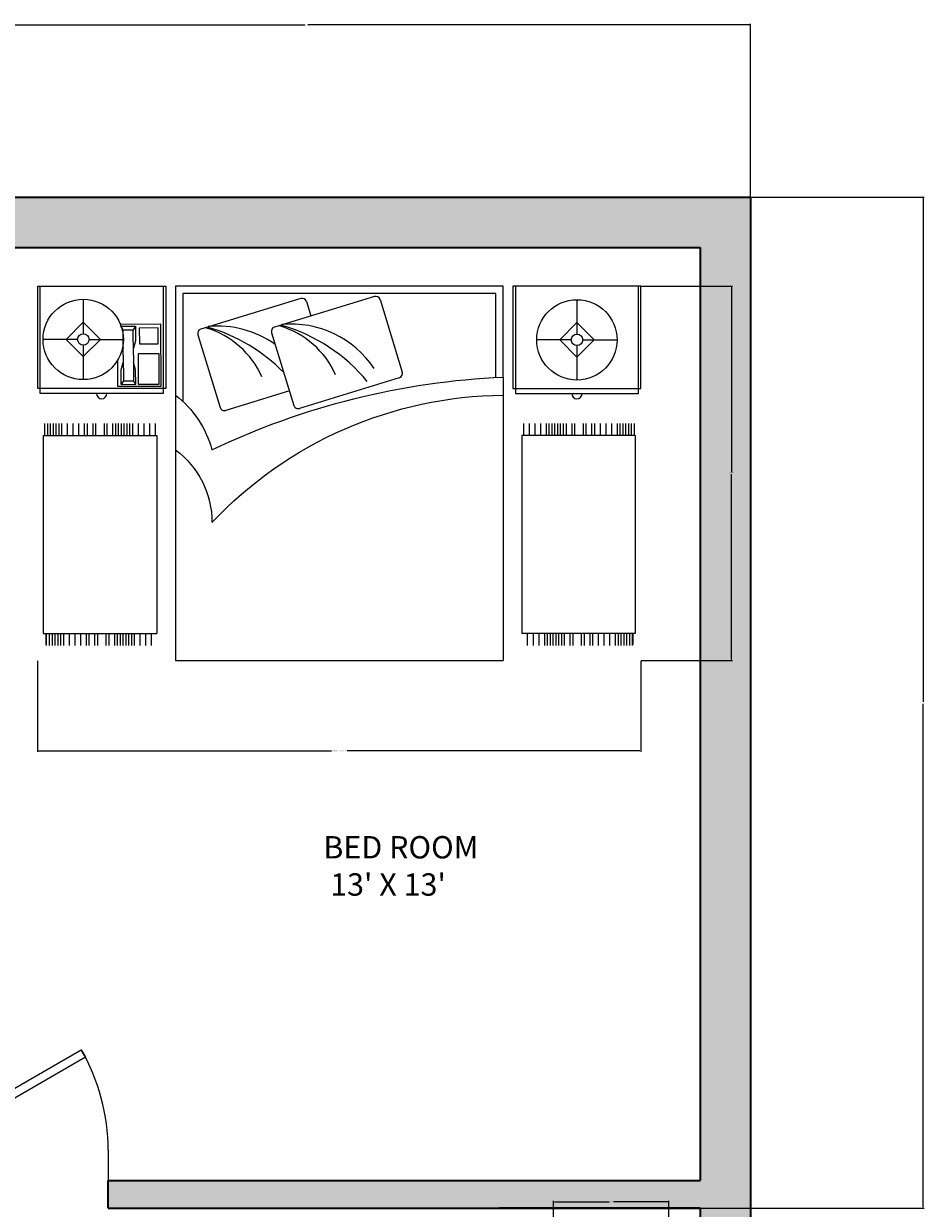
# Model space of a CAD drawing. Units: inches. Extents: x -30 to 437, y -29 to 647.
# Tile 15 of 15: x 276 to 437, y 435 to 647. Entities that reach past the tile are written whole.
import ezdxf

# ---------------------------------------------------------------- set-up
doc = ezdxf.new("R2010")
doc.units = ezdxf.units.IN
doc.header["$MEASUREMENT"] = 0
for name, color, linetype, lineweight in [('A-ANNO-DIMS', 2, 'Continuous', 18), ('A-AREA-IDEN', 7, 'Continuous', 18), ('A-WALL', 7, 'Continuous', 35), ('bedroom', 120, 'Continuous', 18), ('doors', 40, 'Continuous', 25)]:
    doc.layers.add(name, color=color, linetype=linetype, lineweight=lineweight)
doc.layers.add('A-WALL-PATT', color=251, linetype='Continuous', lineweight=13, true_color=0x636466)
doc.styles.get("Standard").update_dxf_attribs({"font": 'arial.ttf'})
doc.dimstyles.get("Standard").update_dxf_attribs({"dimtxt": 0.18, "dimasz": 0.18, "dimexe": 0.18, "dimexo": 0.0625, "dimgap": 0.09, "dimtad": 0, "dimtih": 1, "dimtoh": 1, "dimdec": 4, "dimzin": 0, "dimdsep": 46, "dimtxsty": 'Standard', "dimcen": 0.09, "dimadec": 0, "dimazin": 0, "dimtfac": 1, "dimtdec": 4, "dimtofl": 0, "dimtmove": 0, "dimatfit": 3, "dimfxl": 1, "dimtolj": 1, "dimtzin": 0, "dimarcsym": 0})

# ---------------------------------------------------------------- blocks, each defined once
blk = doc.blocks.new('3')
for p, q in [((185.8665, 224.6766), (185.8665, 225.2363)), ((185.8665, 225.2363), (186.566, 225.2363)), ((185.8805, 224.6487), (185.8805, 225.2363)), ((186.552, 225.2363), (186.552, 224.6487)), ((186.566, 225.2363), (186.566, 224.6766)), ((186.6199, 225.2363), (186.6199, 224.6399)), ((188.4089, 225.2363), (186.6199, 225.2363)), ((188.4089, 224.7393), (188.4089, 225.2363)), ((188.4627, 225.2363), (188.4627, 224.6766)), ((189.1623, 225.2363), (188.4627, 225.2363)), ((188.4767, 225.2363), (188.4767, 224.6486)), ((189.1483, 224.6486), (189.1483, 225.2363)), ((189.1623, 224.6766), (189.1623, 225.2363)), ((186.1157, 225.1643), (186.1157, 224.9763)), ((187.3034, 225.1683), (186.7581, 225.0015)), ((187.7059, 225.1793), (187.1607, 225.0124)), ((187.737, 225.1628), (187.8585, 224.7657)), ((188.8125, 225.1618), (188.8125, 224.9738)), ((187.3344, 225.1518), (187.3586, 225.073)), ((186.0216, 224.9449), (186.1157, 225.0389)), ((186.1157, 225.0389), (186.2097, 224.9449)), ((188.8125, 225.0365), (188.7185, 224.9424)), ((188.9065, 224.9424), (188.8125, 225.0365)), ((186.5397, 225.0274), (186.3193, 225.0266)), ((186.3215, 225.0167), (186.4008, 225.017)), ((186.3334, 224.9969), (186.3215, 225.0167)), ((186.3334, 224.9969), (186.389, 224.9971)), ((186.334, 224.858), (186.3334, 224.9969)), ((186.4008, 225.017), (186.389, 224.9971)), ((186.3895, 224.8582), (186.389, 224.9971)), ((186.4008, 225.017), (186.4011, 224.9376)), ((186.5409, 224.6901), (186.5397, 225.0274)), ((186.7416, 224.9704), (186.8631, 224.5734)), ((187.1442, 224.9814), (187.2657, 224.5843)), ((186.0843, 224.9449), (185.8963, 224.9449)), ((186.1157, 224.8509), (186.0216, 224.9449)), ((186.2097, 224.9449), (186.1157, 224.8509)), ((186.1157, 224.9136), (186.1157, 224.7256)), ((186.147, 224.9449), (186.335, 224.9449)), ((186.3314, 224.9055), (186.3338, 224.8977)), ((186.4011, 224.9376), (186.3894, 224.8979)), ((188.7812, 224.9424), (188.5931, 224.9424)), ((188.7185, 224.9424), (188.8125, 224.8484)), ((188.8125, 224.8484), (188.9065, 224.9424)), ((188.8125, 224.9111), (188.8125, 224.723)), ((188.8438, 224.9424), (189.0319, 224.9424)), ((186.334, 224.858), (186.3345, 224.7191)), ((186.3895, 224.8582), (186.39, 224.7193)), ((186.3023, 224.8297), (186.3029, 224.6892)), ((186.3224, 224.7786), (186.3341, 224.8183)), ((186.3227, 224.6992), (186.3224, 224.7786)), ((186.4017, 224.7789), (186.3897, 224.8185)), ((186.402, 224.6995), (186.4017, 224.7789)), ((186.3345, 224.7191), (186.3227, 224.6992)), ((186.3345, 224.7191), (186.39, 224.7193)), ((186.402, 224.6995), (186.39, 224.7193)), ((187.842, 224.7347), (187.2967, 224.5678)), ((188.4089, 224.7393), (188.4089, 223.1907)), ((186.566, 224.6766), (185.8665, 224.6766)), ((186.552, 224.6487), (185.8805, 224.6487)), ((186.3029, 224.6892), (186.5409, 224.6901)), ((186.3227, 224.6992), (186.402, 224.6995)), ((187.2416, 224.6632), (186.8942, 224.5569)), ((188.4627, 224.6766), (189.1623, 224.6766)), ((188.4767, 224.6486), (189.1483, 224.6486)), ((186.6199, 224.6399), (186.6199, 223.1907)), ((185.904, 224.4849, -0.9094), (185.904, 224.4204, -0.9094)), ((185.9195, 224.4849, -0.9094), (185.9195, 224.4204, -0.9094)), ((185.9195, 224.4849, -0.9094), (185.9195, 224.4204, -0.9094)), ((185.935, 224.4849, -0.9094), (185.935, 224.4204, -0.9094)), ((185.9505, 224.4849, -0.9094), (185.9505, 224.4204, -0.9094)), ((185.966, 224.4849, -0.9094), (185.966, 224.4204, -0.9094)), ((185.9815, 224.4849, -0.9094), (185.9815, 224.4204, -0.9094)), ((185.997, 224.4849, -0.9094), (185.997, 224.4204, -0.9094)), ((186.028, 224.4849, -0.9094), (186.028, 224.4204, -0.9094)), ((186.059, 224.4849, -0.9094), (186.059, 224.4204, -0.9094)), ((186.09, 224.4849, -0.9094), (186.09, 224.4204, -0.9094)), ((186.09, 224.4849, -0.9094), (186.09, 224.4204, -0.9094)), ((186.121, 224.4849, -0.9094), (186.121, 224.4204, -0.9094)), ((186.1365, 224.4849, -0.9094), (186.1365, 224.4204, -0.9094)), ((186.1675, 224.4849, -0.9094), (186.1675, 224.4204, -0.9094)), ((186.183, 224.4849, -0.9094), (186.183, 224.4204, -0.9094)), ((186.2295, 224.4849, -0.9094), (186.2295, 224.4204, -0.9094)), ((186.245, 224.4849, -0.9094), (186.245, 224.4204, -0.9094)), ((186.276, 224.4849, -0.9094), (186.276, 224.4204, -0.9094)), ((186.2915, 224.4849, -0.9094), (186.2915, 224.4204, -0.9094)), ((186.307, 224.4849, -0.9094), (186.307, 224.4204, -0.9094)), ((186.3225, 224.4849, -0.9094), (186.3225, 224.4204, -0.9094)), ((186.338, 224.4849, -0.9094), (186.338, 224.4204, -0.9094)), ((186.3535, 224.4849, -0.9094), (186.3535, 224.4204, -0.9094)), ((186.369, 224.4849, -0.9094), (186.369, 224.4204, -0.9094)), ((186.3845, 224.4849, -0.9094), (186.3845, 224.4204, -0.9094)), ((186.4155, 224.4849, -0.9094), (186.4155, 224.4204, -0.9094)), ((186.4465, 224.4849, -0.9094), (186.4465, 224.4204, -0.9094)), ((186.4775, 224.4849, -0.9094), (186.4775, 224.4204, -0.9094)), ((186.5085, 224.4849, -0.9094), (186.5085, 224.4204, -0.9094)), ((188.5202, 224.4849, -0.9094), (188.5202, 224.4204, -0.9094)), ((188.5512, 224.4849, -0.9094), (188.5512, 224.4204, -0.9094)), ((188.5822, 224.4849, -0.9094), (188.5822, 224.4204, -0.9094)), ((188.6132, 224.4849, -0.9094), (188.6132, 224.4204, -0.9094)), ((188.6442, 224.4849, -0.9094), (188.6442, 224.4204, -0.9094)), ((188.6597, 224.4849, -0.9094), (188.6597, 224.4204, -0.9094)), ((188.6752, 224.4849, -0.9094), (188.6752, 224.4204, -0.9094)), ((188.6907, 224.4849, -0.9094), (188.6907, 224.4204, -0.9094)), ((188.7062, 224.4849, -0.9094), (188.7062, 224.4204, -0.9094)), ((188.7217, 224.4849, -0.9094), (188.7217, 224.4204, -0.9094)), ((188.7372, 224.4849, -0.9094), (188.7372, 224.4204, -0.9094)), ((188.7527, 224.4849, -0.9094), (188.7527, 224.4204, -0.9094)), ((188.7837, 224.4849, -0.9094), (188.7837, 224.4204, -0.9094)), ((188.7992, 224.4849, -0.9094), (188.7992, 224.4204, -0.9094)), ((188.8457, 224.4849, -0.9094), (188.8457, 224.4204, -0.9094)), ((188.8612, 224.4849, -0.9094), (188.8612, 224.4204, -0.9094)), ((188.8922, 224.4849, -0.9094), (188.8922, 224.4204, -0.9094)), ((188.9077, 224.4849, -0.9094), (188.9077, 224.4204, -0.9094)), ((188.9387, 224.4849, -0.9094), (188.9387, 224.4204, -0.9094)), ((188.9387, 224.4849, -0.9094), (188.9387, 224.4204, -0.9094)), ((188.9697, 224.4849, -0.9094), (188.9697, 224.4204, -0.9094)), ((189.0007, 224.4849, -0.9094), (189.0007, 224.4204, -0.9094)), ((189.0317, 224.4849, -0.9094), (189.0317, 224.4204, -0.9094)), ((189.0472, 224.4849, -0.9094), (189.0472, 224.4204, -0.9094)), ((189.0627, 224.4849, -0.9094), (189.0627, 224.4204, -0.9094)), ((189.0782, 224.4849, -0.9094), (189.0782, 224.4204, -0.9094)), ((189.0937, 224.4849, -0.9094), (189.0937, 224.4204, -0.9094)), ((189.1092, 224.4849, -0.9094), (189.1092, 224.4204, -0.9094)), ((189.1092, 224.4849, -0.9094), (189.1092, 224.4204, -0.9094)), ((189.1247, 224.4849, -0.9094), (189.1247, 224.4204, -0.9094)), ((185.8974, 224.4204, -0.9094), (185.8974, 223.3378, -0.9094)), ((185.8974, 224.4204, -0.9094), (186.5174, 224.4204, -0.9094)), ((186.5174, 224.4204, -0.9094), (186.5174, 223.3378, -0.9094)), ((189.1313, 224.4204, -0.9094), (188.5113, 224.4204, -0.9094)), ((188.5113, 224.4204, -0.9094), (188.5113, 223.3378, -0.9094)), ((189.1313, 224.4204, -0.9094), (189.1313, 223.3378, -0.9094)), ((185.8974, 223.3378, -0.9094), (186.5174, 223.3378, -0.9094)), ((185.9114, 223.3378, -0.9094), (185.9114, 223.2789, -0.9094)), ((185.9114, 223.3378, -0.9094), (185.9114, 223.2789, -0.9094)), ((185.9114, 223.3378, -0.9094), (185.9114, 223.2789, -0.9094)), ((185.9138, 223.3378, -0.9094), (185.9138, 223.2732, -0.9094)), ((185.9293, 223.3378, -0.9094), (185.9293, 223.2732, -0.9094)), ((185.9293, 223.3378, -0.9094), (185.9293, 223.2732, -0.9094)), ((185.9448, 223.3378, -0.9094), (185.9448, 223.2732, -0.9094)), ((185.9603, 223.3378, -0.9094), (185.9603, 223.2732, -0.9094)), ((185.9758, 223.3378, -0.9094), (185.9758, 223.2732, -0.9094)), ((185.9913, 223.3378, -0.9094), (185.9913, 223.2732, -0.9094)), ((186.0068, 223.3378, -0.9094), (186.0068, 223.2732, -0.9094)), ((186.0378, 223.3378, -0.9094), (186.0378, 223.2732, -0.9094)), ((186.0688, 223.3378, -0.9094), (186.0688, 223.2732, -0.9094)), ((186.0998, 223.3378, -0.9094), (186.0998, 223.2732, -0.9094)), ((186.0998, 223.3378, -0.9094), (186.0998, 223.2732, -0.9094)), ((186.1308, 223.3378, -0.9094), (186.1308, 223.2732, -0.9094)), ((186.1463, 223.3378, -0.9094), (186.1463, 223.2732, -0.9094)), ((186.1773, 223.3378, -0.9094), (186.1773, 223.2732, -0.9094)), ((186.1928, 223.3378, -0.9094), (186.1928, 223.2732, -0.9094)), ((186.2393, 223.3378, -0.9094), (186.2393, 223.2732, -0.9094)), ((186.2548, 223.3378, -0.9094), (186.2548, 223.2732, -0.9094)), ((186.2858, 223.3378, -0.9094), (186.2858, 223.2732, -0.9094)), ((186.3013, 223.3378, -0.9094), (186.3013, 223.2732, -0.9094)), ((186.3168, 223.3378, -0.9094), (186.3168, 223.2732, -0.9094)), ((186.3323, 223.3378, -0.9094), (186.3323, 223.2732, -0.9094)), ((186.3478, 223.3378, -0.9094), (186.3478, 223.2732, -0.9094)), ((186.3633, 223.3378, -0.9094), (186.3633, 223.2732, -0.9094)), ((186.3788, 223.3378, -0.9094), (186.3788, 223.2732, -0.9094)), ((186.3943, 223.3378, -0.9094), (186.3943, 223.2732, -0.9094)), ((186.4253, 223.3378, -0.9094), (186.4253, 223.2732, -0.9094)), ((186.4563, 223.3378, -0.9094), (186.4563, 223.2732, -0.9094)), ((186.4873, 223.3378, -0.9094), (186.4873, 223.2732, -0.9094)), ((189.1313, 223.3378, -0.9094), (188.5113, 223.3378, -0.9094)), ((188.5414, 223.3378, -0.9094), (188.5414, 223.2732, -0.9094)), ((188.5724, 223.3378, -0.9094), (188.5724, 223.2732, -0.9094)), ((188.6034, 223.3378, -0.9094), (188.6034, 223.2732, -0.9094)), ((188.6344, 223.3378, -0.9094), (188.6344, 223.2732, -0.9094)), ((188.6499, 223.3378, -0.9094), (188.6499, 223.2732, -0.9094)), ((188.6654, 223.3378, -0.9094), (188.6654, 223.2732, -0.9094)), ((188.6809, 223.3378, -0.9094), (188.6809, 223.2732, -0.9094)), ((188.6964, 223.3378, -0.9094), (188.6964, 223.2732, -0.9094)), ((188.7119, 223.3378, -0.9094), (188.7119, 223.2732, -0.9094)), ((188.7274, 223.3378, -0.9094), (188.7274, 223.2732, -0.9094)), ((188.7429, 223.3378, -0.9094), (188.7429, 223.2732, -0.9094)), ((188.7739, 223.3378, -0.9094), (188.7739, 223.2732, -0.9094)), ((188.7894, 223.3378, -0.9094), (188.7894, 223.2732, -0.9094)), ((188.8359, 223.3378, -0.9094), (188.8359, 223.2732, -0.9094)), ((188.8514, 223.3378, -0.9094), (188.8514, 223.2732, -0.9094)), ((188.8824, 223.3378, -0.9094), (188.8824, 223.2732, -0.9094)), ((188.8979, 223.3378, -0.9094), (188.8979, 223.2732, -0.9094)), ((188.9289, 223.3378, -0.9094), (188.9289, 223.2732, -0.9094)), ((188.9289, 223.3378, -0.9094), (188.9289, 223.2732, -0.9094)), ((188.9599, 223.3378, -0.9094), (188.9599, 223.2732, -0.9094)), ((188.9909, 223.3378, -0.9094), (188.9909, 223.2732, -0.9094)), ((189.022, 223.3378, -0.9094), (189.022, 223.2732, -0.9094)), ((189.0375, 223.3378, -0.9094), (189.0375, 223.2732, -0.9094)), ((189.053, 223.3378, -0.9094), (189.053, 223.2732, -0.9094)), ((189.0685, 223.3378, -0.9094), (189.0685, 223.2732, -0.9094)), ((189.084, 223.3378, -0.9094), (189.084, 223.2732, -0.9094)), ((189.0995, 223.3378, -0.9094), (189.0995, 223.2732, -0.9094)), ((189.0995, 223.3378, -0.9094), (189.0995, 223.2732, -0.9094)), ((189.115, 223.3378, -0.9094), (189.115, 223.2732, -0.9094)), ((189.1173, 223.3378, -0.9094), (189.1173, 223.2789, -0.9094)), ((189.1173, 223.3378, -0.9094), (189.1173, 223.2789, -0.9094)), ((189.1173, 223.3378, -0.9094), (189.1173, 223.2789, -0.9094)), ((186.6199, 223.1907), (188.4089, 223.1907))]:
    blk.add_line(p, q)
blk.add_lwpolyline([(188.3691, 224.7374), (188.3691, 225.1965), (186.6596, 225.1965), (186.6596, 224.606)])
for points in [[(186.4217, 225.0072), (186.422, 224.9199), (186.5252, 224.9202), (186.5249, 225.0075)], [(186.4153, 224.8663), (186.4159, 224.6996), (186.531, 224.7), (186.5304, 224.8667)]]:
    blk.add_lwpolyline(points, close=True)
for points in [[(186.6199, 224.6399, -0.162278), (186.8186, 224.3418, -0.100664), (188.4089, 224.7393, -0.100664)], [(186.6199, 224.3418, -0.236068), (186.8186, 223.9442, -0.205258), (188.4089, 224.6399, -0.205258)]]:
    blk.add_lwpolyline(points, format="xyb")
for centre, radius in [((186.1157, 224.9449), 0.2194), ((188.8125, 224.9424), 0.2194), ((186.1157, 224.9449), 0.0313), ((188.8125, 224.9424), 0.0313)]:
    blk.add_circle(centre, radius)
for centre, radius, start, end in [((187.3107, 225.1446), 0.0248, 17.0142, 107.0142), ((187.7132, 225.1555), 0.0248, 17.0142, 107.0142), ((186.7654, 224.9777), 0.0248, 107.0142, 197.0142), ((186.6474, 224.5408), 0.4873, 24.22087, 73.06906), ((186.8477, 224.4712), 0.5468, 54.68511, 95.16051), ((186.5359, 224.1054), 0.9426, 44.27274, 73.71889), ((187.1679, 224.9887), 0.0248, 107.0142, 197.0142), ((187.0499, 224.5517), 0.4873, 24.22087, 73.06906), ((187.2502, 224.4821), 0.5468, 33.78007, 95.16051), ((186.9385, 224.1164), 0.9426, 39.40233, 73.71889), ((187.8347, 224.7585), 0.0248, 287.0142, 17.0142), ((186.2163, 224.6487), 0.028, 180, 0), ((188.8125, 224.6486), 0.028, 180, 0), ((187.2894, 224.5916), 0.0248, 197.0142, 287.0142), ((186.8869, 224.5806), 0.0248, 197.0142, 287.0142)]:
    blk.add_arc(centre, radius, start, end)
blk = doc.blocks.new('*U6')
for p, q in [((0, 0), (0, -6)), ((40, 0), (40, -6))]:
    blk.add_line(p, q)
blk.add_lwpolyline([(0, 0), (34.64, 20), (35.52, 18.48), (0.87, -1.52)], close=True)
blk.add_arc((0, 0), 40, 0, 30)
blk = doc.blocks.new('*D11')
at = {"layer": 'A-ANNO-DIMS', "color": 0, "lineweight": -2, "transparency": 16777216}
for p, q in [((278.06, 532.56), (278.06, 516.24)), ((386.06, 532.56), (386.06, 516.24)), ((278.24, 516.42), (330.68, 516.42)), ((385.88, 516.42), (333.45, 516.42))]:
    blk.add_line(p, q, dxfattribs=at)
at = {"layer": 'A-ANNO-DIMS', "color": 0, "transparency": 16777216}
for points in [[(278.24, 516.45), (278.24, 516.39), (278.06, 516.42)], [(385.88, 516.45), (385.88, 516.39), (386.06, 516.42)]]:
    blk.add_solid(points, dxfattribs=at)
at = {"layer": 'Defpoints', "color": 0, "transparency": 16777216}
for p in [(278.06, 532.62), (386.06, 532.62), (386.06, 516.42)]:
    blk.add_point(p, dxfattribs=at)
at = {"layer": 'A-ANNO-DIMS', "color": 0, "transparency": 16777216, "insert": (332.06, 516.42), "char_height": 0.18, "attachment_point": 5}
blk.add_mtext('\\A1;BED GROUP 108 TYP.', dxfattribs=at)
blk = doc.blocks.new('*D12')
at = {"layer": 'A-ANNO-DIMS', "color": 0, "lineweight": -2, "transparency": 16777216}
for p, q in [((386.12, 599.65), (402.44, 599.65)), ((402.26, 599.47), (402.26, 566.32)), ((402.26, 532.8), (402.26, 565.95)), ((386.12, 532.62), (402.44, 532.62))]:
    blk.add_line(p, q, dxfattribs=at)
at = {"layer": 'A-ANNO-DIMS', "color": 0, "transparency": 16777216}
for points in [[(402.23, 599.47), (402.29, 599.47), (402.26, 599.65)], [(402.23, 532.8), (402.29, 532.8), (402.26, 532.62)]]:
    blk.add_solid(points, dxfattribs=at)
at = {"layer": 'Defpoints', "color": 0, "transparency": 16777216}
for p in [(386.06, 599.65), (402.26, 599.65), (386.06, 532.62)]:
    blk.add_point(p, dxfattribs=at)
at = {"layer": 'A-ANNO-DIMS', "color": 0, "transparency": 16777216, "insert": (402.26, 566.14), "char_height": 0.18, "attachment_point": 5}
blk.add_mtext('\\A1;67 TYP.', dxfattribs=at)
blk = doc.blocks.new('*D29')
at = {"layer": 'A-ANNO-DIMS', "color": 0, "lineweight": -2, "transparency": 16777216}
for p, q in [((246.67, 606.61), (246.67, 646.63)), ((246.85, 646.45), (325.89, 646.45)), ((405.49, 646.45), (326.45, 646.45)), ((405.67, 615.61), (405.67, 646.63))]:
    blk.add_line(p, q, dxfattribs=at)
at = {"layer": 'A-ANNO-DIMS', "color": 0, "transparency": 16777216}
for points in [[(246.85, 646.48), (246.85, 646.42), (246.67, 646.45)], [(405.49, 646.48), (405.49, 646.42), (405.67, 646.45)]]:
    blk.add_solid(points, dxfattribs=at)
at = {"layer": 'Defpoints', "color": 0, "transparency": 16777216}
for p in [(405.67, 646.45), (405.67, 615.55), (246.67, 606.55)]:
    blk.add_point(p, dxfattribs=at)
at = {"layer": 'A-ANNO-DIMS', "color": 0, "transparency": 16777216, "insert": (326.17, 646.45), "char_height": 0.18, "attachment_point": 5}
blk.add_mtext('\\A1;159', dxfattribs=at)
blk = doc.blocks.new('*D40')
at = {"layer": 'A-ANNO-DIMS', "color": 0, "lineweight": -2, "transparency": 16777216}
for p, q in [((405.74, 615.55), (436.75, 615.55)), ((436.57, 615.37), (436.57, 525.23)), ((436.57, 434.73), (436.57, 524.87)), ((396.74, 434.55), (436.75, 434.55))]:
    blk.add_line(p, q, dxfattribs=at)
at = {"layer": 'A-ANNO-DIMS', "color": 0, "transparency": 16777216}
for points in [[(436.54, 615.37), (436.6, 615.37), (436.57, 615.55)], [(436.54, 434.73), (436.6, 434.73), (436.57, 434.55)]]:
    blk.add_solid(points, dxfattribs=at)
at = {"layer": 'Defpoints', "color": 0, "transparency": 16777216}
for p in [(405.67, 615.55), (436.57, 615.55), (396.67, 434.55)]:
    blk.add_point(p, dxfattribs=at)
at = {"layer": 'A-ANNO-DIMS', "color": 0, "transparency": 16777216, "insert": (436.57, 525.05), "char_height": 0.18, "attachment_point": 5}
blk.add_mtext('\\A1;181', dxfattribs=at)
blk = doc.blocks.new('*D47')
at = {"layer": 'A-ANNO-DIMS', "color": 0, "lineweight": -2, "transparency": 16777216}
for p, q in [((370.39, 404.84), (370.39, 435.86)), ((370.57, 435.68), (380.34, 435.68)), ((390.89, 435.68), (381.13, 435.68)), ((391.07, 404.84), (391.07, 435.86))]:
    blk.add_line(p, q, dxfattribs=at)
at = {"layer": 'A-ANNO-DIMS', "color": 0, "transparency": 16777216}
for points in [[(370.57, 435.71), (370.57, 435.65), (370.39, 435.68)], [(390.89, 435.71), (390.89, 435.65), (391.07, 435.68)]]:
    blk.add_solid(points, dxfattribs=at)
at = {"layer": 'Defpoints', "color": 0, "transparency": 16777216}
for p in [(391.07, 435.68), (370.39, 404.78), (391.07, 404.78)]:
    blk.add_point(p, dxfattribs=at)
at = {"layer": 'A-ANNO-DIMS', "color": 0, "transparency": 16777216, "insert": (380.73, 435.68), "char_height": 0.18, "attachment_point": 5}
blk.add_mtext('\\A1;20.68', dxfattribs=at)

msp = doc.modelspace()

# ---------------------------------------------------------------- hatches: boundary and pattern name
at = {"layer": 'A-WALL-PATT'}
h = msp.add_hatch(color=256, dxfattribs=at)
h.dxf.hatch_style = 1
h.paths.add_polyline_path([(393.6054, 183.2352), (369.6054, 183.2352), (369.6054, 213.2352), (393.6054, 213.2352), (393.6054, 207.2352), (394.6054, 207.2352), (394.6054, 211.2352), (395.6054, 211.2352), (395.6054, 185.2352), (394.6054, 185.2352), (394.6054, 189.2352), (393.6054, 189.2352)], flags=0)
h.paths.add_polyline_path([(384.6054, 189.2352, -1), (390.6054, 189.2352, -1)], flags=0)
h.paths.add_polyline_path([(385.6054, 189.2352, -1), (389.6054, 189.2352, -1)], flags=0)
h.paths.add_polyline_path([(374.6054, 189.2352, -1), (382.6054, 189.2352, -1)], flags=0)
h.paths.add_polyline_path([(386.6054, 189.2352, -1), (388.6054, 189.2352, -1)], flags=0)
h.paths.add_polyline_path([(375.6054, 189.2352, -1), (381.6054, 189.2352, -1)], flags=0)
h.paths.add_polyline_path([(376.6054, 189.2352, -1), (380.6054, 189.2352, -1)], flags=0)
h.paths.add_polyline_path([(377.6054, 189.2352, -1), (379.6054, 189.2352, -1)], flags=0)
h.paths.add_polyline_path([(390.6054, 195.2352), (374.6054, 195.2352), (374.6054, 201.2352), (390.6054, 201.2352)], flags=0)
h.paths.add_polyline_path([(389.6054, 196.2352), (375.6054, 196.2352), (375.6054, 200.2352), (389.6054, 200.2352)], flags=0)
h.paths.add_polyline_path([(383.6054, 207.2352, -1), (391.6054, 207.2352, -1)], flags=0)
h.paths.add_polyline_path([(384.6054, 207.2352, -1), (390.6054, 207.2352, -1)], flags=0)
h.paths.add_polyline_path([(385.6054, 207.2352, -1), (389.6054, 207.2352, -1)], flags=0)
h.paths.add_polyline_path([(386.6054, 207.2352, -1), (388.6054, 207.2352, -1)], flags=0)
h.paths.add_polyline_path([(375.6054, 207.2352, -1), (381.6054, 207.2352, -1)], flags=0)
h.paths.add_polyline_path([(376.6054, 207.2352, -1), (380.6054, 207.2352, -1)], flags=0)
h.paths.add_polyline_path([(377.6054, 207.2352, -1), (379.6054, 207.2352, -1)], flags=0)
h.paths.add_polyline_path([(305.5437, 160.3663, -0.41421356), (304.0437, 158.8663), (271.0437, 158.8663, -0.41421356), (269.5437, 160.3663), (269.5437, 178.3663, -0.41421356), (271.0437, 179.8663), (304.0437, 179.8663, -0.41421356), (305.5437, 178.3663)], flags=0)
h.paths.add_polyline_path([(304.0437, 165.3663, -0.41421356), (303.0437, 164.3663), (289.2937, 164.3663, -0.41421356), (288.2937, 165.3663), (288.2937, 177.3663, -0.41421356), (289.2937, 178.3663), (303.0437, 178.3663, -0.41421356), (304.0437, 177.3663)], flags=0)
h.paths.add_polyline_path([(296.5437, 171.3663, -1), (295.5437, 171.3663, -1)], flags=0)
h.paths.add_polyline_path([(286.7937, 165.3663, -0.41421356), (285.7937, 164.3663), (272.0437, 164.3663, -0.41421356), (271.0437, 165.3663), (271.0437, 177.3663, -0.41421356), (272.0437, 178.3663), (285.7937, 178.3663, -0.41421356), (286.7937, 177.3663)], flags=0)
h.paths.add_polyline_path([(279.5437, 171.3663, -1), (278.5437, 171.3663, -1)], flags=0)
h.paths.add_polyline_path([(360.6737, 290.5474), (360.6737, 300.5474), (396.6737, 300.5474), (396.6737, 290.5474)], flags=0)
h.paths.add_polyline_path([(259.6737, 124.5474), (259.6737, 114.5474), (171.6737, 114.5474), (171.6737, 124.5474)], flags=0)
h.paths.add_polyline_path([(288.0737, 215.3705), (286.7097, 214.583), (268.7097, 245.7599), (270.0737, 246.5474)], flags=0)
h.paths.add_polyline_path([(259.6737, 168.5474), (256.6737, 168.5474), (256.6737, 173.5474), (256.6737, 179.0224), (255.8753, 177.6395), (224.2956, 195.872, 0.12053744), (220.1737, 179.0224, 0.12053744), (216.0518, 195.872), (184.4721, 177.6395), (183.6737, 179.0224), (215.2836, 197.2724), (216.0821, 195.8895), (216.0518, 195.872, -0.12053744), (220.1737, 179.0224, -0.12053744), (224.2956, 195.872), (224.2653, 195.8895), (225.0638, 197.2724), (256.6737, 179.0224), (256.6737, 173.5474), (259.6737, 173.5474)], flags=0)
h.paths.add_polyline_path([(386.7943, 325.4601), (372.6871, 325.4601), (372.6871, 339.5673), (386.7943, 339.5673)], flags=0)
h.paths.add_polyline_path([(359.5875, 343.7429), (357.7905, 343.7429), (357.7905, 327.9179), (359.3933, 327.9179, 0.41420885), (361.5302, 330.0549), (361.5302, 341.8434, 0.41436161)], flags=0)
h.paths.add_polyline_path([(341.7887, 323.1235, -0.11921667), (340.7839, 323.1235)], flags=0)
h.paths.add_polyline_path([(379.6332, 328.8632), (379.6332, 332.2699), (376.0992, 332.2699, 0.39427733)], flags=0)
h.paths.add_polyline_path([(375.5299, 332.459, -1), (383.8511, 332.459, -1)], flags=0)
h.paths.add_polyline_path([(388.9363, 344.7425), (372.5309, 344.7425, -0.41421356), (370.394, 346.8794), (370.394, 347.5594, -0.39085173), (372.3472, 349.7005, -0.43951011), (370.394, 351.4933), (370.394, 365.1894, -0.40305452), (372.2191, 367.1298, -0.41839453), (370.394, 368.9291), (370.394, 382.6251, -0.40885826), (372.2519, 384.5722, -0.42377324), (370.394, 386.3707), (370.394, 400.0667, -0.38660687), (372.1327, 402.0094), (372.531, 402.0094, -0.41421834), (370.394, 404.1464), (370.394, 404.7778, -0.41420891), (372.5309, 406.9147), (388.9363, 406.9147, -0.41421821), (391.0733, 404.7778), (391.0733, 346.8794, -0.41421356)], flags=0)
edge = h.paths.add_edge_path(flags=0)
edge.add_spline(control_points=[(349.3585, 363.204), (349.0859, 363.204), (348.8133, 363.2227), (348.2712, 363.2973), (348.0016, 363.3531), (347.3533, 363.5328), (346.9776, 363.6755), (346.2445, 364.0308), (345.887, 364.2432), (345.1953, 364.7329), (344.8611, 365.0101), (344.2197, 365.6237), (343.9125, 365.9603), (343.211, 366.8336), (342.8313, 367.3965), (342.1401, 368.6117), (341.8286, 369.2641), (341.2807, 370.64), (341.0443, 371.3636), (340.6522, 372.8619), (340.4964, 373.6367), (340.2695, 375.2158), (340.1983, 376.0203), (340.142, 377.6365), (340.157, 378.4483), (340.2729, 380.0567), (340.3738, 380.8533), (340.6589, 382.4093), (340.8432, 383.1686), (341.2906, 384.629), (341.5538, 385.3301), (342.1531, 386.6544), (342.4891, 387.2776), (343.2266, 388.4288), (343.6281, 388.9567), (344.4879, 389.9012), (344.9463, 390.3178), (345.7981, 390.9428), (346.182, 391.1771), (346.9712, 391.5648), (347.3766, 391.7182), (348.2004, 391.9387), (348.6189, 392.0058), (349.4588, 392.0508), (349.8801, 392.0288), (350.7146, 391.8966), (351.1278, 391.7865), (351.9366, 391.4822), (352.3323, 391.2882), (353.0989, 390.8223), (353.4699, 390.5504), (354.1819, 389.9355), (354.5229, 389.5924), (355.1706, 388.8418), (355.4772, 388.4343), (356.1315, 387.4422), (356.4671, 386.8397), (357.0692, 385.5581), (357.3356, 384.879), (357.7933, 383.4624), (357.9846, 382.725), (358.2875, 381.2112), (358.3992, 380.4349), (358.5404, 378.8643), (358.5699, 378.0699), (358.546, 376.4841), (358.4926, 375.6928), (358.3042, 374.1343), (358.1692, 373.3672), (357.8207, 371.8774), (357.6072, 371.1549), (357.1067, 369.7735), (356.8196, 369.1148), (356.1782, 367.8787), (355.8238, 367.3013), (355.0551, 366.244), (354.6408, 365.7641), (353.7607, 364.9161), (353.2948, 364.5481), (352.445, 364.0149), (352.0701, 363.822), (351.3034, 363.5117), (350.9116, 363.3943), (350.1325, 363.2418), (349.7455, 363.204), (349.3585, 363.204)], knot_values=[3.14159265, 3.14159265, 3.14159265, 3.14159265, 3.22691715, 3.22691715, 3.31224165, 3.31224165, 3.43426671, 3.43426671, 3.55629177, 3.55629177, 3.67831683, 3.67831683, 3.8003419, 3.8003419, 3.97157384, 3.97157384, 4.14280577, 4.14280577, 4.31403771, 4.31403771, 4.48526965, 4.48526965, 4.65650159, 4.65650159, 4.82773353, 4.82773353, 4.99896547, 4.99896547, 5.1701974, 5.1701974, 5.34142934, 5.34142934, 5.51266128, 5.51266128, 5.68389322, 5.68389322, 5.85512516, 5.85512516, 5.98669107, 5.98669107, 6.11825699, 6.11825699, 6.24982291, 6.24982291, 6.38138882, 6.38138882, 6.51295474, 6.51295474, 6.64452065, 6.64452065, 6.77608657, 6.77608657, 6.90765249, 6.90765249, 7.0392184, 7.0392184, 7.20701563, 7.20701563, 7.37481286, 7.37481286, 7.54261009, 7.54261009, 7.71040732, 7.71040732, 7.87820455, 7.87820455, 8.04600178, 8.04600178, 8.21379901, 8.21379901, 8.38159624, 8.38159624, 8.54939347, 8.54939347, 8.7171907, 8.7171907, 8.88498794, 8.88498794, 9.05278517, 9.05278517, 9.17820699, 9.17820699, 9.30362881, 9.30362881, 9.42477796, 9.42477796, 9.42477796, 9.42477796], degree=3, periodic=0)
edge.add_line((341.1696, 384.3006), (341.2012, 384.2808))
edge = h.paths.add_edge_path(flags=0)
edge.add_line((344.3353, 388.7801), (344.317, 388.7915))
edge.add_ellipse((349.3585, 377.6204), major_axis=(0, -13.7895), ratio=0.62186025, start_angle=-244.867444, end_angle=-124.769923)
h.paths.add_polyline_path([(163.6737, 163.1474), (132.4968, 145.1474), (131.7093, 146.5114), (162.8862, 164.5114)], flags=0)
h.paths.add_polyline_path([(366.4355, 409.0896, -0.41423669), (364.2985, 406.9525, -0.4913499), (361.5302, 408.8973), (361.5302, 420.6405, 0.41421356), (359.3932, 422.7775), (357.7905, 422.7775), (357.7905, 406.9525), (359.6317, 406.9525, 0.42741026), (361.5332, 408.9757, 0.39869469), (363.6672, 406.9525, 0.51958103), (366.4355, 409.0895)], flags=0)
h.paths.add_polyline_path([(386.7943, 410.9671), (372.6871, 410.9671), (372.6871, 425.0742), (386.7943, 425.0742)], flags=0)
h.paths.add_polyline_path([(379.6332, 414.3701), (379.6332, 417.7768), (376.0992, 417.7768, 0.39427733)], flags=0)
h.paths.add_polyline_path([(375.5299, 417.966, -1), (383.8511, 417.966, -1)], flags=0)
h.paths.add_polyline_path([(150.0377, 351.583), (148.6737, 352.3705), (166.6737, 383.5474), (168.0377, 382.7599)], flags=0)
h.paths.add_polyline_path([(91.6737, 234.1974), (66.559, 219.6974), (65.9246, 220.7962), (91.0393, 235.2962)], flags=0)
h.paths.add_polyline_path([(255.4612, 443.5834), (254.6737, 444.9474), (285.8506, 462.9474), (286.6381, 461.5834)], flags=0)
h.paths.add_polyline_path([(176.2737, 394.5474), (158.2737, 425.7243), (159.6377, 426.5118), (177.6377, 395.3349)], flags=0)
h.paths.add_polyline_path([(243.6737, 439.5474), (243.0393, 438.4486), (217.9246, 452.9486), (218.559, 454.0474)], flags=0)
h.paths.add_polyline_path([(38.1264, 269.8429), (40.2408, 269.8429), (40.2408, 270.3508), (38.1264, 270.3508)], flags=0)
h.paths.add_polyline_path([(75.7157, 289.9439), (40.2408, 289.9439), (38.1264, 289.6524), (40.2408, 289.6524)], flags=0)
h.paths.add_polyline_path([(75.7157, 270.0846), (77.6447, 270.0846), (77.6697, 270.1626), (75.7175, 270.1626)], flags=0)
h.paths.add_polyline_path([(80.5373, 293.3002), (33.0467, 293.3002), (13.5054, 293.3002), (13.5054, 351.9244), (29.7898, 351.9244), (80.5373, 351.9244)], flags=0)
h.paths.add_polyline_path([(46.0261, 212.466, -0.50131678), (27.1651, 207.5106), (21.165, 209.5107), (21.165, 206.5107), (22.665, 206.5107), (22.665, 203.5107), (21.165, 203.5107), (21.165, 203.0107), (13.165, 203.0107), (13.165, 224.0107), (21.165, 224.0107), (21.165, 217.5107), (27.1649, 219.5106, -0.50132349), (46.0261, 214.5554, -0.13289091)], flags=0)
h.paths.add_polyline_path([(44.688, 211.8666, -0.48007965), (27.165, 209.5107), (27.165, 217.5107, -0.4800795), (44.688, 215.1547, -0.21500378)], flags=0)
h.paths.add_polyline_path([(19.415, 204.0107), (15.165, 204.0107, -0.41421356), (14.165, 204.7607), (14.165, 222.0107, -0.41421356), (14.915, 223.0107), (19.165, 223.0107, -0.41421356), (20.165, 222.2607), (20.165, 205.0107, -0.41421356)], flags=0)
h.paths.add_polyline_path([(32.7608, 269.0719), (31.8439, 269.0719), (31.8439, 268.6134), (13.5054, 268.6134), (13.5054, 291.5366), (31.8439, 291.5366), (32.7608, 291.0781), (32.7608, 280.9919, -1), (32.7608, 279.1581)], flags=0)
h.paths.add_polyline_path([(40.2408, 360.1436), (38.1264, 360.1436), (38.1264, 359.6357), (40.2408, 359.6357)], flags=0)
h.paths.add_polyline_path([(75.7157, 355.2807), (40.2408, 355.2807), (38.1264, 355.5722), (40.2408, 355.5722), (40.2408, 355.2807), (75.7157, 355.2807), (75.7157, 375.5982), (40.2408, 375.5982), (38.1264, 375.3817), (40.2408, 375.3817), (40.2408, 375.5982), (75.7157, 375.5982), (77.9733, 375.062), (75.7175, 375.062), (75.7175, 374.554)], flags=0)
h.paths.add_polyline_path([(42.8174, 299.814, 0.13867074), (34.1602, 294.603), (14.8081, 294.603), (14.8081, 350.6216), (29.8539, 350.6216, 0.09822056)], flags=0)
h.paths.add_polyline_path([(15.8636, 276.7781, -0.30640166), (20.3757, 283.4499), (20.3483, 290.6726), (31.4014, 290.7146), (31.4309, 282.9124), (26.8287, 282.895, -0.26006276), (30.241, 276.7781, -1)], flags=0)
h.paths.add_polyline_path([(26.1332, 276.7781), (23.0523, 273.6972), (19.9714, 276.7781), (23.0523, 279.8589), (23.0523, 283.9209), (21.3493, 283.9145), (20.7006, 283.5219), (20.6907, 286.1226), (23.2914, 286.1325), (25.8936, 285.7522), (27.1939, 285.7572), (28.4928, 286.1522), (31.0935, 286.1621), (31.0918, 286.6172), (25.6303, 286.5965), (25.616, 290.3675), (31.0775, 290.3882), (31.0918, 286.6172), (31.1034, 283.5614), (28.5027, 283.5515), (25.9005, 283.9317), (23.0523, 283.9209), (23.0523, 279.8589)], flags=0)
h.paths.add_polyline_path([(24.0793, 276.7781, -1), (22.0253, 276.7781, -1)], flags=0)
h.paths.add_polyline_path([(35.7687, 302.2895, -0.41421356), (35.2283, 301.2726), (22.2164, 297.2909, -0.41421356), (21.1995, 297.8313), (15.7317, 315.6996, -0.41421356), (16.2721, 316.7165), (18.8554, 317.507), (15.3721, 328.8904, -0.41421356), (15.9125, 329.9073), (28.9244, 333.889, -0.41421356), (29.9414, 333.3486), (35.4091, 315.4802, -0.41421356), (34.8687, 314.4633), (32.2854, 313.6728)], flags=0)
h.paths.add_polyline_path([(361.3728, 532.6207), (302.7487, 532.6207), (302.7487, 580.1113), (302.7487, 599.6527), (361.3728, 599.6527), (361.3728, 583.3682)], flags=0)
h.paths.add_polyline_path([(370.1, 575.0316), (370.1, 572.9172), (370.6079, 572.9172), (370.6079, 575.0316)], flags=0)
h.paths.add_polyline_path([(385.0466, 537.4423), (385.0466, 572.9172), (384.8302, 575.0316), (384.8302, 572.9172)], flags=0)
h.paths.add_polyline_path([(384.5104, 535.3262), (384.5104, 537.4406), (384.0025, 537.4406), (364.7291, 537.4423), (364.7291, 572.9172), (365.0206, 575.0316), (365.0206, 572.9172), (364.7291, 572.9172), (364.7291, 537.4423), (384.5884, 537.4423), (384.5884, 535.5133)], flags=0)
h.paths.add_polyline_path([(384.5884, 535.5133), (383.4945, 535.164), (383.4945, 537.4406), (382.9866, 535.3262), (382.9866, 537.4406), (383.4945, 535.3262), (383.4945, 537.4406), (384.5884, 537.4406)], flags=0)
h.paths.add_polyline_path([(23.874, 286.8174), (21.0132, 286.8065), (21.0004, 290.1875), (23.8612, 290.1983)], flags=0)
h.paths.add_polyline_path([(242.9824, 511.1667), (234.9824, 511.1667), (234.9824, 517.6667), (228.9825, 515.6667, -0.50132349), (210.1213, 520.622, -0.13289091), (210.1213, 522.7114, -0.50131678), (228.9823, 527.6667), (234.9824, 525.6667), (234.9824, 528.6667), (233.4824, 528.6667), (233.4824, 531.6667), (234.9824, 531.6667), (234.9824, 532.1667), (242.9824, 532.1667)], flags=0)
h.paths.add_polyline_path([(236.9824, 512.1667, -0.41421356), (235.9824, 512.9167), (235.9824, 530.1667, -0.41421356), (236.7324, 531.1667), (240.9824, 531.1667, -0.41421356), (241.9824, 530.4167), (241.9824, 513.1667, -0.41421356), (241.2324, 512.1667)], flags=0)
h.paths.add_polyline_path([(279.533, 537.4423), (279.533, 535.5133), (279.6111, 535.4884), (279.6111, 537.4406)], flags=0)
h.paths.add_polyline_path([(279.2913, 575.0316), (279.2913, 572.9172), (279.7992, 572.9172), (279.7992, 575.0316)], flags=0)
h.paths.add_polyline_path([(211.4594, 520.0227, -0.21500378), (211.4594, 523.3107, -0.48007965), (228.9824, 525.6667), (228.9824, 517.6667, -0.4800795)], flags=0)
h.paths.add_polyline_path([(32.7627, 354.1465), (31.8457, 354.1465), (31.8457, 353.688), (13.5054, 353.688), (13.5054, 376.6134), (31.8457, 376.6134), (32.7627, 376.1549), (32.7627, 366.0677, -1), (32.7627, 364.2337)], flags=0)
h.paths.add_polyline_path([(15.9446, 365.1507, -1), (30.3234, 365.1507, -1)], flags=0)
h.paths.add_polyline_path([(41.213, 428.467), (43.3274, 428.467), (43.3274, 428.9749), (41.213, 428.9749)], flags=0)
h.paths.add_polyline_path([(78.8022, 448.568), (43.3274, 448.568), (41.213, 448.2765), (43.3274, 448.2765)], flags=0)
h.paths.add_polyline_path([(78.8022, 428.7087), (80.7313, 428.7087), (80.7562, 428.7868), (78.804, 428.7868)], flags=0)
h.paths.add_polyline_path([(26.2152, 365.1507), (23.134, 362.0696), (20.0529, 365.1507), (23.134, 368.2319)], flags=0)
h.paths.add_polyline_path([(24.1611, 365.1507, -1), (22.107, 365.1507, -1)], flags=0)
h.paths.add_polyline_path([(309.2625, 570.3406, 0.13867074), (304.0514, 578.9978), (304.0514, 598.3499), (360.07, 598.3499), (360.07, 583.3041, 0.09822056)], flags=0)
h.paths.add_polyline_path([(246.6737, 552.5474), (129.6737, 552.5474), (129.6737, 606.5474), (246.6737, 606.5474)], flags=16)
h.paths.add_polyline_path([(373.6822, 580.3953), (363.595, 580.3953), (363.595, 581.3123), (363.1365, 581.3123), (363.1365, 599.6527), (386.0619, 599.6527), (386.0619, 581.3123), (385.6034, 580.3953), (375.5162, 580.3953, -1)], flags=0)
h.paths.add_polyline_path([(83.6239, 451.9244), (36.1333, 451.9244), (16.5919, 451.9244), (16.5919, 510.5485), (32.8764, 510.5485), (83.6239, 510.5485)], flags=0)
h.paths.add_polyline_path([(367.4098, 590.024, -1), (381.7886, 590.024, -1)], flags=0)
h.paths.add_polyline_path([(374.5992, 586.9428), (371.518, 590.024), (374.5992, 593.1052), (377.6803, 590.024)], flags=0)
h.paths.add_polyline_path([(373.5721, 590.024, -1), (375.6262, 590.024, -1)], flags=0)
h.paths.add_polyline_path([(324.9287, 577.7489, -0.41421356), (323.9118, 578.2893), (323.1212, 580.8726), (311.7379, 577.3893, -0.41421356), (310.721, 577.9297), (306.7393, 590.9416, -0.41421356), (307.2797, 591.9585), (325.1481, 597.4263, -0.41421356), (326.165, 596.8859), (326.9555, 594.3026), (338.3388, 597.7859, -0.41421356), (339.3557, 597.2455), (343.3374, 584.2336, -0.41421356), (342.797, 583.2167)], flags=0)
h.paths.add_polyline_path([(300.5265, 580.3972), (290.4404, 580.3972, -1), (288.6065, 580.3972), (278.5203, 580.3972), (278.5203, 581.3142), (278.0619, 581.3142), (278.0619, 599.6527), (300.985, 599.6527), (300.985, 581.3142)], flags=0)
h.paths.add_polyline_path([(300.163, 581.7567), (292.3609, 581.7271), (292.3434, 586.3294, -0.75567924), (279.0378, 590.1057, -0.82536731), (292.8983, 592.7823), (300.1211, 592.8097)], flags=0)
h.paths.add_polyline_path([(299.8367, 582.0805), (296.0656, 582.0662), (293.0098, 582.0546), (292.9999, 584.6553), (293.3802, 587.2575), (293.3694, 590.1057), (289.3074, 590.1057), (286.2265, 587.0248), (283.1456, 590.1057), (286.2265, 593.1866), (289.3074, 590.1057), (293.3694, 590.1057), (293.3629, 591.8088), (292.9703, 592.4575), (295.5711, 592.4673), (295.5809, 589.8666), (295.2007, 587.2644), (295.2056, 585.9641), (295.6006, 584.6652), (295.6105, 582.0645), (296.0656, 582.0662), (296.0449, 587.5277), (299.8159, 587.542)], flags=0)
h.paths.add_polyline_path([(285.1995, 590.1057, -1), (287.2535, 590.1057, -1)], flags=0)
h.paths.add_polyline_path([(299.6467, 589.2969), (296.2658, 589.284), (296.255, 592.1448), (299.6359, 592.1576)], flags=0)
h.paths.add_polyline_path([(35.8473, 427.696), (34.9304, 427.696), (34.9304, 427.2376), (16.5919, 427.2376), (16.5919, 450.1607), (34.9304, 450.1607), (35.8473, 449.7022), (35.8473, 439.6161, -1), (35.8473, 437.7822)], flags=0)
h.paths.add_polyline_path([(18.9502, 435.4022, -0.30640166), (23.4623, 442.074), (23.4349, 449.2968), (34.4879, 449.3387), (34.5175, 441.5366), (29.9152, 441.5191, -0.26006276), (33.3275, 435.4022, -1)], flags=0)
h.paths.add_polyline_path([(29.2197, 435.4022), (26.1389, 432.3213), (23.058, 435.4022), (26.1389, 438.4831), (26.1389, 442.5451), (24.4358, 442.5386), (23.7871, 442.1461), (23.7772, 444.7468), (26.378, 444.7566), (28.9801, 444.3764), (30.2805, 444.3813), (31.5794, 444.7764), (34.1801, 444.7862), (34.1784, 445.2413), (28.7169, 445.2206), (28.7026, 448.9917), (34.164, 449.0124), (34.1784, 445.2413), (34.1899, 442.1855), (31.5892, 442.1756), (28.987, 442.5559), (26.1389, 442.5451), (26.1389, 438.4831)], flags=0)
h.paths.add_polyline_path([(27.1658, 435.4022, -1), (25.1119, 435.4022, -1)], flags=0)
h.paths.add_polyline_path([(45.904, 458.4382, 0.13867074), (37.2467, 453.2271), (17.8947, 453.2271), (17.8947, 509.2457), (32.9405, 509.2457, 0.09822056)], flags=0)
h.paths.add_polyline_path([(26.9605, 445.4415), (24.0997, 445.4307), (24.0869, 448.8116), (26.9477, 448.8225)], flags=0)
h.paths.add_polyline_path([(38.3149, 459.8967), (25.3029, 455.915, -0.41421356), (24.286, 456.4554), (18.8183, 474.3238, -0.41421356), (19.3586, 475.3407), (21.942, 476.1312), (18.4587, 487.5145, -0.41421356), (18.999, 488.5314), (32.011, 492.5131, -0.41421356), (33.0279, 491.9727), (38.4957, 474.1044, -0.41421356), (37.9553, 473.0875), (35.3719, 472.297), (38.8553, 460.9136, -0.41421356)], flags=0)
h.paths.add_polyline_path([(43.3274, 518.7678), (41.213, 518.7678), (41.213, 518.2598), (43.3274, 518.2598)], flags=0)
h.paths.add_polyline_path([(78.8022, 513.9049), (43.3274, 513.9049), (41.213, 514.1964), (43.3274, 514.1964), (43.3274, 513.9049), (78.8022, 513.9049), (78.8022, 534.2223), (43.3274, 534.2223), (41.213, 534.0059), (43.3274, 534.0059), (43.3274, 534.2223), (78.8022, 534.2223), (81.0599, 533.6861), (78.804, 533.6861), (78.804, 533.1782)], flags=0)
h.paths.add_polyline_path([(121.6737, 556.8974), (121.0393, 555.7986), (95.9246, 570.2986), (96.559, 571.3974)], flags=0)
h.paths.add_polyline_path([(35.8493, 512.7707), (34.9322, 512.7707), (34.9322, 512.3122), (16.5919, 512.3122), (16.5919, 535.2376), (34.9322, 535.2376), (35.8493, 534.7791), (35.8493, 524.6919, -1), (35.8493, 522.8579)], flags=0)
h.paths.add_polyline_path([(19.0312, 523.7749, -1), (33.41, 523.7749, -1)], flags=0)
h.paths.add_polyline_path([(26.2206, 520.6937), (23.1394, 523.7749), (26.2206, 526.8561), (29.3018, 523.7749)], flags=0)
h.paths.add_polyline_path([(25.1935, 523.7749, -1), (27.2476, 523.7749, -1)], flags=0)
h.paths.add_polyline_path([(28.4381, 586.0173), (22.438, 588.0173), (22.438, 585.0173), (23.938, 585.0173), (23.938, 582.0173), (22.438, 582.0173), (22.438, 581.5173), (14.438, 581.5173), (14.438, 602.5173), (22.438, 602.5173), (22.438, 596.0173), (28.4379, 598.0173, -0.50132349), (47.2992, 593.062, -0.13289091), (47.2992, 590.9726, -0.50131678)], flags=0)
h.paths.add_polyline_path([(28.438, 588.0174), (28.438, 596.0173, -0.4800795), (45.961, 593.6614, -0.21500378), (45.961, 590.3733, -0.48007965)], flags=0)
h.paths.add_polyline_path([(20.688, 582.5173), (16.438, 582.5173, -0.41421356), (15.438, 583.2673), (15.438, 600.5173, -0.41421356), (16.188, 601.5173), (20.438, 601.5173, -0.41421356), (21.438, 600.7673), (21.438, 583.5173, -0.41421356)], flags=0)
h.paths.add_polyline_path([(171.6737, 2.0474), (171.6737, 104.5474), (259.6737, 104.5474), (259.6737, 148.5474), (396.6737, 148.5474), (396.6737, 2.0474), (405.6737, 2.0474), (405.6737, 615.5474), (1.6737, 615.5474), (1.6737, 2.0474)])
h.paths.add_polyline_path([(171.6737, 104.5474), (259.6737, 104.5474), (259.6737, 210.5474), (264.6737, 210.5474), (264.6737, 153.5474), (396.6737, 153.5474), (396.6737, 249.5474), (264.6737, 249.5474), (264.6737, 246.5474), (259.6737, 246.5474), (259.6737, 254.5474), (396.6737, 254.5474), (396.6737, 434.5474), (290.6737, 434.5474), (290.6737, 439.5474), (396.6737, 439.5474), (396.6737, 606.5474), (251.6737, 606.5474), (251.6737, 439.5474), (254.6737, 439.5474), (254.6737, 434.5474), (243.6737, 434.5474), (243.6737, 439.5474), (246.6737, 439.5474), (246.6737, 547.5474), (186.6737, 547.5474), (186.6737, 439.5474), (214.6737, 439.5474), (214.6737, 434.5474), (186.6737, 434.5474), (186.6737, 430.5474), (181.6737, 430.5474), (181.6737, 547.5474), (121.6737, 547.5474), (121.6737, 552.5474), (124.6737, 552.5474), (124.6737, 606.5474), (10.6737, 606.5474), (10.6737, 552.5474), (92.6737, 552.5474), (92.6737, 547.5474), (10.6737, 547.5474), (10.6737, 391.5474), (181.6737, 391.5474), (181.6737, 394.5474), (186.6737, 394.5474), (186.6737, 386.5474), (171.6737, 386.5474), (171.6737, 383.5474), (166.6737, 383.5474), (166.6737, 386.5474), (10.6737, 386.5474), (10.6737, 238.5474), (62.6737, 238.5474), (62.6737, 233.5474), (10.6737, 233.5474), (10.6737, 173.5474), (94.6737, 173.5474), (94.6737, 233.5474), (91.6737, 233.5474), (91.6737, 238.5474), (166.6737, 238.5474), (166.6737, 347.5474), (171.6737, 347.5474), (171.6737, 233.5474), (99.6737, 233.5474), (99.6737, 173.5474), (127.6737, 173.5474), (127.6737, 168.5474), (10.6737, 168.5474), (10.6737, 11.0474), (166.6737, 11.0474), (166.6737, 168.5474), (163.6737, 168.5474), (163.6737, 173.5474), (183.6737, 173.5474), (183.6737, 168.5474), (171.6737, 168.5474)])

# ---------------------------------------------------------------- linework, layer by layer
at = {"layer": 'A-WALL'}
for p, q in [((251.6737, 606.5474), (396.6737, 606.5474)), ((396.6737, 606.5474), (396.6737, 439.5474)), ((290.6737, 439.5474), (396.6737, 439.5474)), ((290.6737, 434.5474), (290.6737, 439.5474)), ((290.6737, 434.5474), (396.6737, 434.5474)), ((396.6737, 434.5474), (360.6737, 434.5474)), ((396.6737, 434.5474), (396.6737, 254.5474))]:
    msp.add_line(p, q, dxfattribs=at)
msp.add_lwpolyline([(171.6737, 2.0474), (1.6737, 2.0474), (1.6737, 615.5474), (405.6737, 615.5474), (405.6737, 2.0474), (396.6737, 2.0474)], dxfattribs=at)

# ---------------------------------------------------------------- block references
at = {"layer": 'bedroom', "xscale": 32.76894482774335, "yscale": 32.76894482774335, "zscale": 32.76894482774335}
msp.add_blockref('3', (-5812.5871, -6781.1022), dxfattribs=at)
at = {"layer": 'doors', "xscale": 0.8999999999999548, "yscale": 0.8999999999999548, "zscale": 0.8999999999999548}
msp.add_blockref('*U6', (254.6737, 444.9474), dxfattribs=at)

# ---------------------------------------------------------------- texts
at = {"layer": 'A-AREA-IDEN', "insert": (327.9755, 501.1843), "char_height": 4, "attachment_point": 1}
msp.add_mtext_dynamic_manual_height_columns(" BED ROOM\\P  13' X 13'", width=58.79004, gutter_width=1, heights=[0], dxfattribs=at)

# ---------------------------------------------------------------- dimensions: what is measured, and where the dimension line sits
at = {"layer": 'A-ANNO-DIMS'}
for base, p1, p2, override, picture, middle in [((405.6737, 646.4474), (246.6737, 606.5474), (405.6737, 615.5474), {"dimdec": 0, "dimlfac": 1, "dimrnd": 0, "dimzin": 0, "dimdsep": 46, "dimlunit": 2}, '*D29', (326.1737, 646.4474)), ((391.0733, 435.6778), (370.394, 404.7778), (391.0733, 404.7778), {"dimdec": 2, "dimlfac": 1, "dimrnd": 0, "dimzin": 0, "dimdsep": 46, "dimlunit": 2}, '*D47', (380.7336, 435.6778))]:
    dim = msp.add_linear_dim(base=base, p1=p1, p2=p2, dimstyle='Standard', override=override, dxfattribs=at)
    dim.commit()
    dim.dimension.update_dxf_attribs({"geometry": picture, "text_midpoint": middle})
dim = msp.add_linear_dim(base=(436.5737, 615.5474), p1=(396.6737, 434.5474), p2=(405.6737, 615.5474), angle=90, dimstyle='Standard', override={"dimdec": 0, "dimlfac": 1, "dimrnd": 0, "dimzin": 0, "dimdsep": 46, "dimlunit": 2}, dxfattribs=at)
dim.commit()
dim.dimension.update_dxf_attribs({"geometry": '*D40', "text_midpoint": (436.5737, 525.0474)})
dim = msp.add_linear_dim(base=(402.2619, 599.6527), p1=(386.0619, 532.6207), p2=(386.0619, 599.6527), angle=90, text='<> TYP.', dimstyle='Standard', override={"dimdec": 0, "dimlfac": 1, "dimrnd": 0, "dimzin": 0, "dimdsep": 46, "dimlunit": 2}, dxfattribs=at)
dim.commit()
dim.dimension.update_dxf_attribs({"geometry": '*D12', "text_midpoint": (402.2619, 566.1367)})
dim = msp.add_linear_dim(base=(386.0619, 516.4207), p1=(278.0619, 532.6207), p2=(386.0619, 532.6207), text='BED GROUP <> TYP.', dimstyle='Standard', override={"dimdec": 0, "dimlfac": 1, "dimrnd": 0, "dimzin": 0, "dimdsep": 46, "dimlunit": 2}, dxfattribs=at)
dim.commit()
dim.dimension.update_dxf_attribs({"geometry": '*D11', "text_midpoint": (332.0619, 516.4207)})

doc.saveas('drawing.dxf')
